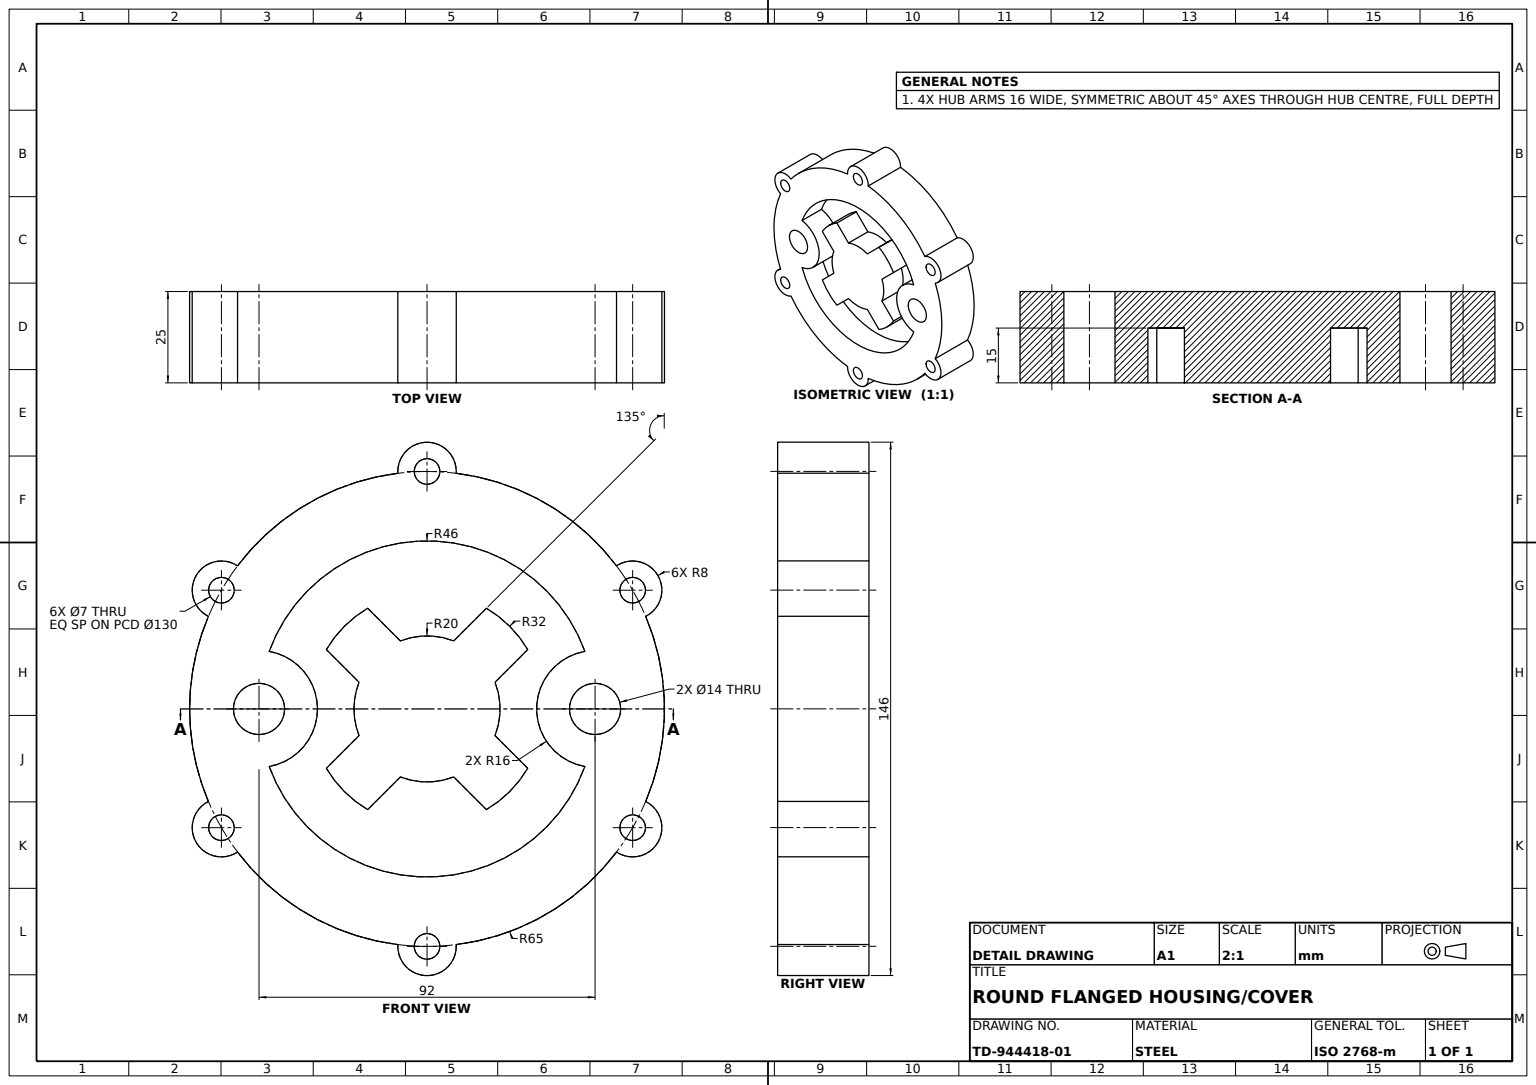
from build123d import *

# Parameters (mm, degrees)
FLANGE_PROFILE_SKETCH_R   = 3.5
FLANGE_BODY_25MM_DEPTH    = 25
THROUGH_HOLES_SKETCH_R    = 7
THROUGH_HOLES_DEPTH       = 25
ANNULAR_POCKET_15MM_DEPTH = 15
CROSS_HUB_15MM_DEPTH      = 15


with BuildPart() as part:
    # Flange Profile Sketch → Flange Body 25mm (new body)
    with BuildSketch(Plane.XY):
        with BuildLine():
            ThreePointArc((-7.984837703, 64.507692308), (-32.5, 56.291651246), (-51.872881427, 39.168918449))
            ThreePointArc((-51.872881427, 39.168918449), (-63.219854476, 36.5), (-59.857719129, 25.338773858))
            ThreePointArc((-59.857719129, 25.338773858), (-65, 0), (-59.857719129, -25.338773858))
            ThreePointArc((-59.857719129, -25.338773858), (-63.219854476, -36.5), (-51.872881427, -39.168918449))
            ThreePointArc((-51.872881427, -39.168918449), (-32.5, -56.291651246), (-7.984837703, -64.507692308))
            ThreePointArc((-7.984837703, -64.507692308), (0, -73), (7.984837703, -64.507692308))
            ThreePointArc((7.984837703, -64.507692308), (32.5, -56.291651246), (51.872881427, -39.168918449))
            ThreePointArc((51.872881427, -39.168918449), (63.219854476, -36.5), (59.857719129, -25.338773858))
            ThreePointArc((59.857719129, -25.338773858), (65, 0), (59.857719129, 25.338773858))
            ThreePointArc((59.857719129, 25.338773858), (63.219854476, 36.5), (51.872881427, 39.168918449))
            ThreePointArc((51.872881427, 39.168918449), (32.5, 56.291651246), (7.984837703, 64.507692308))
            ThreePointArc((7.984837703, 64.507692308), (0, 73), (-7.984837703, 64.507692308))
        make_face()
        with Locations((0, 65)):
            Circle(FLANGE_PROFILE_SKETCH_R, mode=Mode.SUBTRACT)
        with Locations((56.291651246, 32.5)):
            Circle(FLANGE_PROFILE_SKETCH_R, mode=Mode.SUBTRACT)
        with Locations((56.291651246, -32.5)):
            Circle(FLANGE_PROFILE_SKETCH_R, mode=Mode.SUBTRACT)
        with Locations((0, -65)):
            Circle(FLANGE_PROFILE_SKETCH_R, mode=Mode.SUBTRACT)
        with Locations((-56.291651246, -32.5)):
            Circle(FLANGE_PROFILE_SKETCH_R, mode=Mode.SUBTRACT)
        with Locations((-56.291651246, 32.5)):
            Circle(FLANGE_PROFILE_SKETCH_R, mode=Mode.SUBTRACT)
    extrude(amount=FLANGE_BODY_25MM_DEPTH)

    # Through Holes Sketch → Through Holes (cut)
    with BuildSketch(Plane.XY.offset(25)):
        with Locations((46, 0)):
            Circle(THROUGH_HOLES_SKETCH_R)
        with Locations(Location((-46, 0, 0), (0, 0, 180))):
            Circle(THROUGH_HOLES_SKETCH_R)
    extrude(amount=-THROUGH_HOLES_DEPTH, mode=Mode.SUBTRACT)

    # Annular Pocket Sketch → Annular Pocket 15mm (cut)
    with BuildSketch(Plane.XY.offset(25)):
        with BuildLine():
            ThreePointArc((43.217391304, 15.756176213), (0, 46), (-43.217391304, 15.756176213))
            ThreePointArc((-43.217391304, 15.756176213), (-30, 0), (-43.217391304, -15.756176213))
            ThreePointArc((-43.217391304, -15.756176213), (0, -46), (43.217391304, -15.756176213))
            ThreePointArc((43.217391304, -15.756176213), (30, 0), (43.217391304, 15.756176213))
        make_face()
    extrude(amount=-ANNULAR_POCKET_15MM_DEPTH, mode=Mode.SUBTRACT)

    # Cross Hub Sketch → Cross Hub 15mm (add)
    with BuildSketch(Plane.XY.offset(10)):
        with BuildLine():
            Line((-7.304627147, 18.618335646), (-16.252048051, 27.56575655))
            ThreePointArc((-16.252048051, 27.56575655), (-22.627416998, 22.627416998), (-27.56575655, 16.252048051))
            Line((-27.56575655, 16.252048051), (-18.618335646, 7.304627147))
            ThreePointArc((-18.618335646, 7.304627147), (-20, 0), (-18.618335646, -7.304627147))
            Line((-18.618335646, -7.304627147), (-27.56575655, -16.252048051))
            ThreePointArc((-27.56575655, -16.252048051), (-22.627416998, -22.627416998), (-16.252048051, -27.56575655))
            Line((-16.252048051, -27.56575655), (-7.304627147, -18.618335646))
            ThreePointArc((-7.304627147, -18.618335646), (0, -20), (7.304627147, -18.618335646))
            Line((7.304627147, -18.618335646), (16.252048051, -27.56575655))
            ThreePointArc((16.252048051, -27.56575655), (22.627416998, -22.627416998), (27.56575655, -16.252048051))
            Line((27.56575655, -16.252048051), (18.618335646, -7.304627147))
            ThreePointArc((18.618335646, -7.304627147), (20, 0), (18.618335646, 7.304627147))
            Line((18.618335646, 7.304627147), (27.56575655, 16.252048051))
            ThreePointArc((27.56575655, 16.252048051), (22.627416998, 22.627416998), (16.252048051, 27.56575655))
            Line((16.252048051, 27.56575655), (7.304627147, 18.618335646))
            ThreePointArc((7.304627147, 18.618335646), (0, 20), (-7.304627147, 18.618335646))
        make_face()
    extrude(amount=CROSS_HUB_15MM_DEPTH)


solid = part.part
